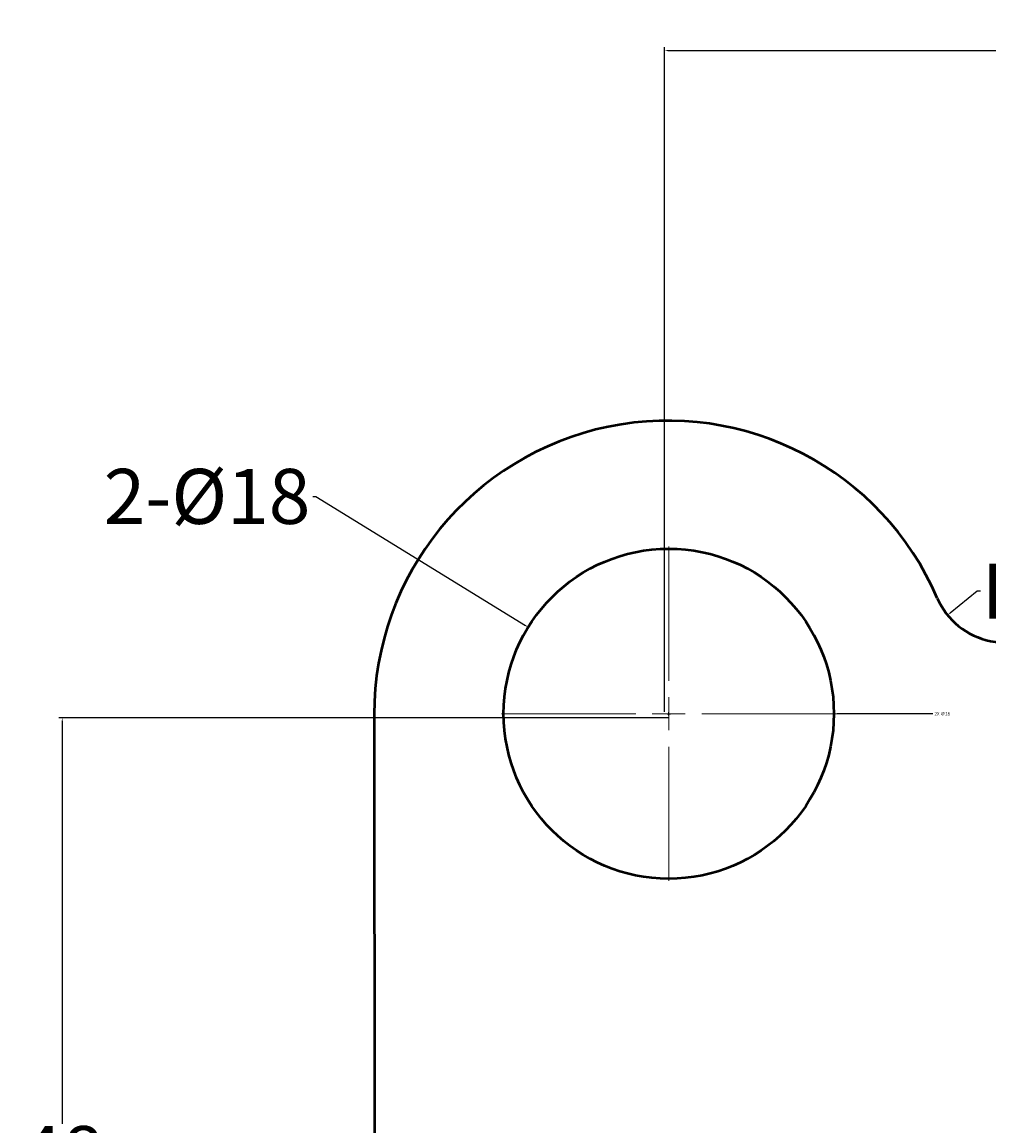
# Model space of a CAD drawing. Units: millimetres. Extents: x -50 to 109, y -46 to 152.
# Tile 11 of 18: x -40 to 13, y 92 to 152. Entities that reach past the tile are written whole.
import ezdxf

# ---------------------------------------------------------------- set-up
doc = ezdxf.new("R2010")
doc.units = ezdxf.units.MM
doc.header["$MEASUREMENT"] = 0
doc.linetypes.add('CENTER', pattern=[50.8, 31.75, -6.35, 6.35, -6.35])
for name, color, linetype, lineweight in [('M-CNTR', 1, 'CENTER', 18), ('M-DIMS', 2, 'Continuous', 25), ('M-OUTL', 7, 'Continuous', 50)]:
    doc.layers.add(name, color=color, linetype=linetype, lineweight=lineweight)
doc.styles.get("Standard").update_dxf_attribs({"font": 'arial.ttf'})
doc.dimstyles.get("Standard").update_dxf_attribs({"dimtxt": 0.18, "dimasz": 0.18, "dimexe": 0.18, "dimexo": 0.0625, "dimgap": 0.09, "dimtad": 0, "dimtih": 1, "dimtoh": 1, "dimdec": 4, "dimzin": 0, "dimdsep": 46, "dimtxsty": 'Standard', "dimcen": 0.09, "dimadec": 0, "dimazin": 0, "dimtfac": 1, "dimtdec": 4, "dimtofl": 0, "dimtmove": 0, "dimatfit": 3, "dimfxl": 1, "dimtolj": 1, "dimtzin": 0, "dimarcsym": 0})

# ---------------------------------------------------------------- blocks, each defined once
blk = doc.blocks.new('*U5')
at = {"layer": 'M-CNTR', "color": 0, "transparency": 16777216}
for p, q in [((0, 1.8), (0, 9.12)), ((-9.12, 0), (-1.8, 0)), ((1.8, 0), (9.12, 0)), ((0, -9.12), (0, -1.8))]:
    blk.add_line(p, q, dxfattribs=at)
at = {"layer": 'M-CNTR', "color": 0, "linetype": 'Continuous', "transparency": 16777216}
for p, q in [((0, -0.9), (0, 0.9)), ((-0.9, 0), (0.9, 0))]:
    blk.add_line(p, q, dxfattribs=at)
blk = doc.blocks.new('*D7')
at = {"layer": 'Defpoints', "color": 0, "transparency": 16777216}
for p in [(70.892, 150.415), (-5.074, 114.299), (70.892, 114.299)]:
    blk.add_point(p, dxfattribs=at)
at = {"layer": 'M-DIMS', "color": 0, "lineweight": -2, "transparency": 16777216}
for p, q in [((-5.074, 114.361), (-5.074, 150.595)), ((70.892, 114.361), (70.892, 150.595)), ((-4.894, 150.415), (30.684, 150.415)), ((70.712, 150.415), (35.134, 150.415))]:
    blk.add_line(p, q, dxfattribs=at)
at = {"layer": 'M-DIMS', "color": 0, "transparency": 16777216}
for points in [[(-4.894, 150.445), (-4.894, 150.385), (-5.074, 150.415)], [(70.712, 150.445), (70.712, 150.385), (70.892, 150.415)]]:
    blk.add_solid(points, dxfattribs=at)
at = {"layer": 'M-DIMS', "color": 0, "transparency": 16777216, "insert": (32.909, 150.415), "char_height": 0.18, "attachment_point": 5}
blk.add_mtext('\\A1;{\\H16.66667x;76}', dxfattribs=at)
blk = doc.blocks.new('*D10')
at = {"layer": 'Defpoints', "color": 0, "transparency": 16777216}
for p in [(13.47, 122.141), (10.357, 119.628)]:
    blk.add_point(p, dxfattribs=at)
at = {"layer": 'M-DIMS', "color": 0, "lineweight": -2, "transparency": 16777216}
for p, q in [((11.974, 120.933), (10.497, 119.741)), ((12.154, 120.933), (11.974, 120.933))]:
    blk.add_line(p, q, dxfattribs=at)
at = {"layer": 'M-DIMS', "color": 0, "transparency": 16777216}
blk.add_solid([(10.478, 119.764), (10.516, 119.718), (10.357, 119.628)], dxfattribs=at)
at = {"layer": 'M-DIMS', "color": 0, "transparency": 16777216, "insert": (14.656, 120.933), "char_height": 0.18, "attachment_point": 5}
blk.add_mtext('\\A1;{\\H16.66667x;R4}', dxfattribs=at)
blk = doc.blocks.new('*D13')
at = {"layer": 'Defpoints', "color": 0, "transparency": 16777216}
for p in [(-12.502, 118.971), (2.821, 109.526)]:
    blk.add_point(p, dxfattribs=at)
at = {"layer": 'M-DIMS', "color": 0, "lineweight": -2, "transparency": 16777216}
for p, q in [((-24.251, 126.101), (-24.071, 126.101)), ((-24.071, 126.101), (-12.655, 119.065)), ((-4.931, 114.248), (-4.751, 114.248)), ((-4.841, 114.158), (-4.841, 114.338))]:
    blk.add_line(p, q, dxfattribs=at)
at = {"layer": 'M-DIMS', "color": 0, "transparency": 16777216}
blk.add_solid([(-12.64, 119.091), (-12.671, 119.04), (-12.502, 118.971)], dxfattribs=at)
at = {"layer": 'M-DIMS', "color": 0, "transparency": 16777216, "insert": (-30.012, 126.101), "char_height": 0.18, "attachment_point": 5}
blk.add_mtext('\\A1;{\\H16.66667x;2-%%C18}', dxfattribs=at)
blk = doc.blocks.new('*D15')
at = {"layer": 'Defpoints', "color": 0, "transparency": 16777216}
for p in [(-4.766, 114.02), (-37.902, 66.508), (-3.772, 66.508)]:
    blk.add_point(p, dxfattribs=at)
at = {"layer": 'M-DIMS', "color": 0, "lineweight": -2, "transparency": 16777216}
for p, q in [((-4.828, 114.02), (-38.082, 114.02)), ((-37.902, 113.84), (-37.902, 91.886)), ((-37.902, 66.688), (-37.902, 88.643)), ((-3.834, 66.508), (-38.082, 66.508))]:
    blk.add_line(p, q, dxfattribs=at)
at = {"layer": 'M-DIMS', "color": 0, "transparency": 16777216}
for points in [[(-37.932, 113.84), (-37.872, 113.84), (-37.902, 114.02)], [(-37.932, 66.688), (-37.872, 66.688), (-37.902, 66.508)]]:
    blk.add_solid(points, dxfattribs=at)
at = {"layer": 'M-DIMS', "color": 0, "transparency": 16777216, "insert": (-37.902, 90.264), "char_height": 0.18, "attachment_point": 5}
blk.add_mtext('\\A1;{\\H16.66667x;48}', dxfattribs=at)
blk = doc.blocks.new('*D31')
at = {"layer": 'Defpoints', "color": 0, "transparency": 16777216}
for p in [(-13.841, 114.249), (4.159, 114.248)]:
    blk.add_point(p, dxfattribs=at)
at = {"layer": 'M-DIMS', "color": 0, "lineweight": -2, "transparency": 16777216}
for p, q in [((-4.931, 114.248), (-4.751, 114.248)), ((-4.841, 114.158), (-4.841, 114.338)), ((9.559, 114.248), (4.339, 114.248))]:
    blk.add_line(p, q, dxfattribs=at)
at = {"layer": 'M-DIMS', "color": 0, "transparency": 16777216}
blk.add_solid([(4.339, 114.278), (4.339, 114.218), (4.159, 114.248)], dxfattribs=at)
at = {"layer": 'M-DIMS', "color": 0, "transparency": 16777216, "insert": (10.067, 114.248), "char_height": 0.18, "attachment_point": 5}
blk.add_mtext('\\A1;2X ∅18', dxfattribs=at)

msp = doc.modelspace()

# ---------------------------------------------------------------- linework, layer by layer
at = {"layer": 'M-OUTL'}
msp.add_line((-20.89964, 114.2123), (-20.84638, 67.15852), dxfattribs=at)
msp.add_circle((-4.8406, 114.24848), 9, dxfattribs=at)
for centre, radius, start, end in [((-4.89965, 114.23041), 16, 23.2974659, 180.0648553), ((13.46962, 122.14051), 4, 203.2974659, 314.6720761)]:
    msp.add_arc(centre, radius, start, end, dxfattribs=at)

# ---------------------------------------------------------------- block references
at = {"layer": 'M-CNTR'}
msp.add_blockref('*U5', (-4.8406, 114.24848), dxfattribs=at)

# ---------------------------------------------------------------- dimensions: what is measured, and where the dimension line sits
at = {"layer": 'M-DIMS'}
dim = msp.add_linear_dim(base=(70.89158, 150.41471), p1=(-5.07376, 114.29893), p2=(70.89158, 114.29893), text='{\\H16.66667x;76}', dimstyle='Standard', override={"dimclrd": 0, "dimclre": 0, "dimclrt": 0}, dxfattribs=at)
dim.commit()
dim.dimension.update_dxf_attribs({"geometry": '*D7', "text_midpoint": (32.90891, 150.41471)})
for p1, p2, text, override, picture, middle in [((2.82105, 109.52628), (-12.50225, 118.97067), '{\\H16.66667x;2-%%C18}', {"dimclrd": 0, "dimclre": 0, "dimclrt": 0}, '*D13', (-30.01162, 126.10102)), ((-13.8406, 114.24895), (4.1594, 114.248), '2X <>', {"dimdec": 0, "dimlfac": 1, "dimrnd": 0, "dimzin": 0, "dimdsep": 46, "dimlunit": 2}, '*D31', (9.5594, 114.24772))]:
    dim = msp.add_diameter_dim_2p(p1=p1, p2=p2, text=text, dimstyle='Standard', override=override, dxfattribs=at)
    dim.commit()
    dim.dimension.update_dxf_attribs({"geometry": picture, "text_midpoint": middle, "dimtype": 163})
dim = msp.add_radius_dim(center=(13.46962, 122.14051), mpoint=(10.35719, 119.62799), text='{\\H16.66667x;R4}', dimstyle='Standard', override={"dimclrd": 0, "dimclre": 0, "dimclrt": 0}, dxfattribs=at)
dim.commit()
dim.dimension.update_dxf_attribs({"geometry": '*D10', "text_midpoint": (14.65628, 120.93283), "dimtype": 164})
dim = msp.add_linear_dim(base=(-37.90219, 66.50813), p1=(-4.76572, 114.02048), p2=(-3.77162, 66.50813), angle=90, text='{\\H16.66667x;48}', dimstyle='Standard', override={"dimclrd": 0, "dimclre": 0, "dimclrt": 0}, dxfattribs=at)
dim.commit()
dim.dimension.update_dxf_attribs({"geometry": '*D15', "text_midpoint": (-37.90219, 90.26431)})

doc.saveas('drawing.dxf')
